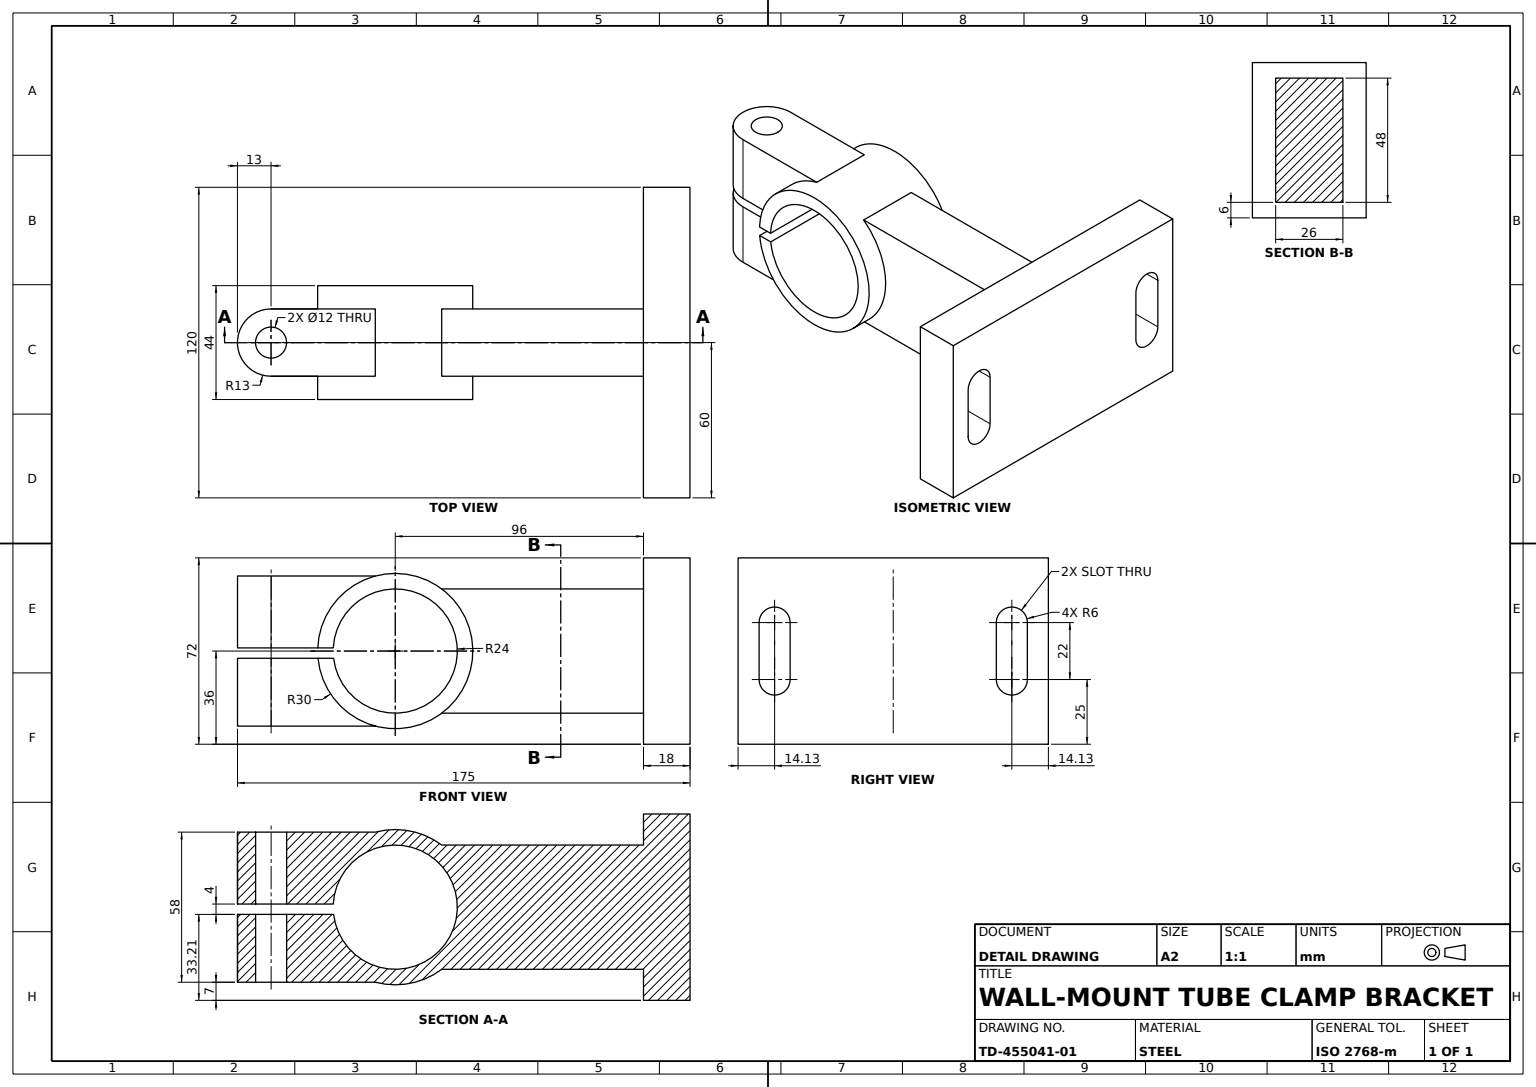
SolidWorks part; units mm, degrees
material "Plain Carbon Steel"
ref_plane "Front Plane" through (0, 0, 0) normal (0, 0, 1) x (1, 0, 0)
ref_plane "Top Plane" through (0, 0, 0) normal (0, 1, 0) x (1, 0, 0)
ref_plane "Right Plane" through (0, 0, 0) normal (1, 0, 0) x (0, 0, -1)
sketch "Base Plate Sketch" plane through (0, 0, 0) normal (0, 0, 1) x (1, 0, 0)
  line L0 (0, 102.1249) -> (0, -110.2738) construction
  line L1 (-181.2486, 0) -> (193.3406, 0) construction
  line L3 (0, 0) -> (120, 0)
  line L4 (0, 0) -> (0, 72)
  line L5 (0, 72) -> (120, 72)
  line L6 (120, 0) -> (120, 72)
  dimension "D1" = 120
  dimension "D2" = 72
extrude "Base Plate 120x72x18" add sketch "Base Plate Sketch" along normal mid plane 18 contours L5 L6 L3 L4
sketch "Arm Profile Sketch" plane through (0, 0, 9) normal (0, 0, 1) x (1, 0, 0)
  line L0 (120, 0) -> (120, 72) construction
  line L1 (47, 60) -> (73, 60)
  line L2 (47, 60) -> (47, 12)
  line L3 (47, 12) -> (73, 12)
  line L4 (73, 60) -> (73, 12)
  line L5 (47, 60) -> (73, 12) construction
  line L6 (47, 12) -> (73, 60) construction
  line L7 (0, 0) -> (120, 0) construction
  point P0 (60, 36)
  dimension "D1" = 47
  dimension "D2" = 36
  dimension "D3" = 26
  dimension "D4" = 48
ref_plane "Plane3" through (60, 0, 0) normal (1, 0, 0) x (0, 0, -1)
sketch "Clamp Ring Sketch" plane through (60, 0, 0) normal (1, 0, 0) x (0, 0, -1)
  line L1 (0, 102.4993) -> (0, -30.6773) construction
  circle A2 centre (-105, 36) radius 30
  circle A3 centre (-105, 36) radius 24
  dimension "D1" = 60
  dimension "D2" = 48
  dimension "D3" = 96
extrude "Clamp Ring" add sketch "Clamp Ring Sketch" along normal mid plane 44 separate body contours A2 | A3
extrude "Arm" add sketch "Arm Profile Sketch" along normal up to surface (78 mm away) contours L1 L4 L3 L2
ref_plane "Plane7" through (60, 0, 0) normal (1, 0, 0) x (0, 0, -1)
sketch "Clamp Lug Sketch" plane through (60, 0, 0) normal (1, 0, 0) x (0, 0, -1)
  line L0 (-153, 7) -> (-153, 65)
  line L2 (-153, 7) -> (-112.6811, 7)
  line L5 (30.8352, 36) -> (-229.6426, 36) construction
  line L6 (-153, 65) -> (-112.6811, 65)
  circle A0 centre (-105, 36) radius 30 construction
  arc A1 (-112.6811, 65) -> (-112.6811, 7) centre (-105, 36) ccw
  dimension "D1" = 58
  dimension "D2" = 48
extrude "Clamp Lug" add sketch "Clamp Lug Sketch" along normal mid plane 26 contours L0 L6 A1 L2
sketch "Clamp Lug Extension Sketch" plane through (0, 7, 0) normal (0, -1, 0) x (1, 0, 0)
  line L0 (73, 153) -> (47, 153) construction
  line L1 (47, 153) -> (73, 153)
  arc A0 (73, 153) -> (47, 153) centre (60, 153) ccw
extrude "Clamp Lug Extension" add sketch "Clamp Lug Extension Sketch" against normal blind 58
sketch "Clamp Bolt Hole Sketch" plane through (0, 7, 0) normal (0, -1, 0) x (1, 0, 0)
  circle A0 centre (60, 153) radius 6
  dimension "D1" = 12
extrude "Clamp Bolt Hole Ø12" cut sketch "Clamp Bolt Hole Sketch" against normal blind 78 contours A0
ref_plane "Plane8" through (0, 0, 166) normal (0, 0, 1) x (1, 0, 0)
sketch "Clamp Split Slot Sketch" plane through (0, 0, 166) normal (0, 0, 1) x (1, 0, 0)
  line L0 (-3.7866, 35.2119) -> (123.7866, 35.2119) construction
  line L1 (38, 66) -> (38, 6) construction
  line L2 (38, 37.2119) -> (82, 37.2119)
  line L3 (38, 37.2119) -> (38, 33.2119)
  line L4 (38, 33.2119) -> (82, 33.2119)
  line L5 (82, 37.2119) -> (82, 33.2119)
  line L6 (38, 37.2119) -> (82, 33.2119) construction
  line L7 (38, 33.2119) -> (82, 37.2119) construction
  line L10 (82, 6) -> (82, 66) construction
  point P2 (60, 35.2119)
  dimension "D1" = 4
  dimension "D2" = 35.2119
extrude "Clamp Split Slot 4mm" cut sketch "Clamp Split Slot Sketch" against normal blind 78
sketch "Mounting Slots Sketch" plane through (0, 0, 9) normal (0, 0, 1) x (1, 0, 0)
  line L0 (14.1324, 47) -> (14.1324, 25) construction
  line L1 (20.1324, 47) -> (20.1324, 25)
  line L2 (8.1324, 47) -> (8.1324, 25)
  line L4 (0, 0) -> (0, 72) construction
  line L7 (60, 85.9046) -> (60, -9.3926) construction
  line L8 (105.8676, 47) -> (105.8676, 25) construction
  line L9 (99.8676, 47) -> (99.8676, 25)
  line L10 (111.8676, 47) -> (111.8676, 25)
  arc A0 (20.1324, 47) -> (8.1324, 47) centre (14.1324, 47) ccw
  arc A1 (8.1324, 25) -> (20.1324, 25) centre (14.1324, 25) ccw
  arc A2 (99.8676, 47) -> (111.8676, 47) centre (105.8676, 47) cw
  arc A3 (111.8676, 25) -> (99.8676, 25) centre (105.8676, 25) cw
  point P2 (14.1324, 36)
  point P11 (0, 36)
  point P15 (105.8676, 36)
  dimension "D2" = 22
  dimension "D1" = 6
  dimension "D3" = 14.1324
  dimension "D4" = 60
extrude "Mounting Slots 2x" cut sketch "Mounting Slots Sketch" against normal blind 78 contours L1 A1 L2 A0 | L10 A3 L9 A2
